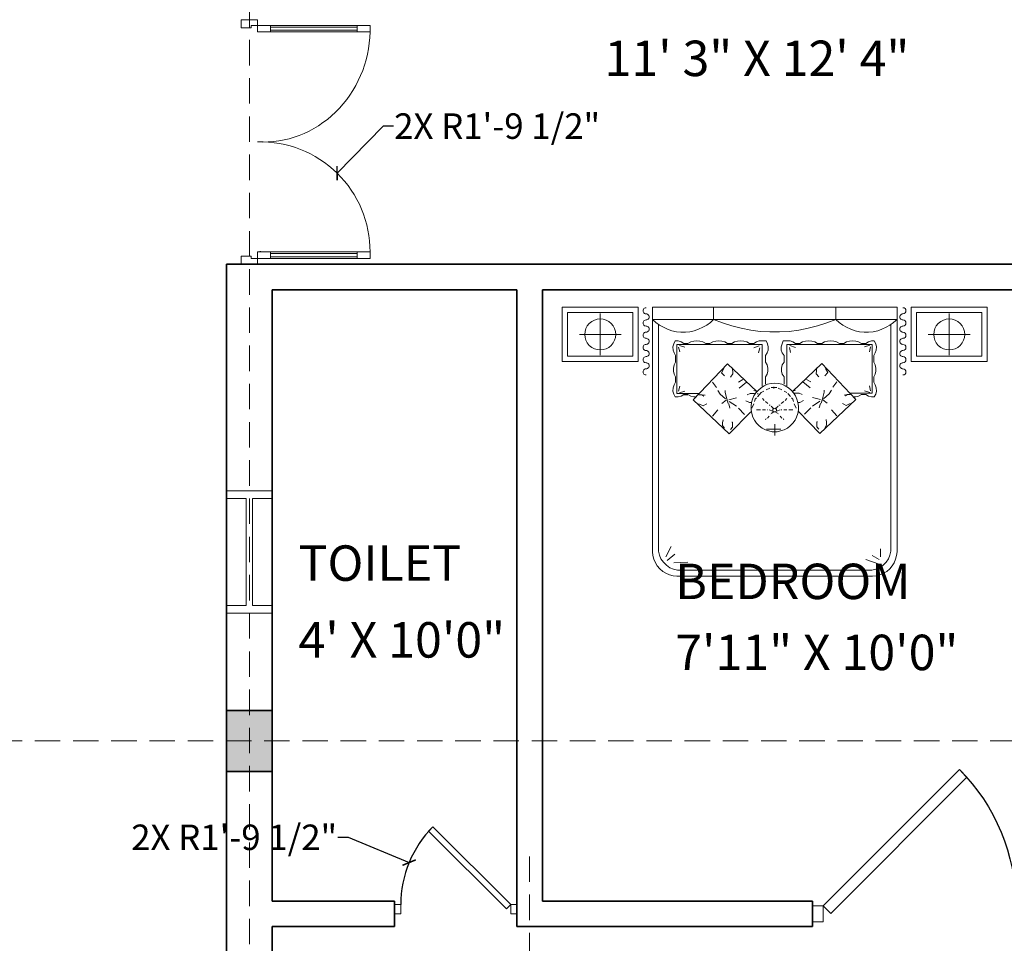
# Model space of a CAD drawing. Units: inches. Extents: x 782 to 2660, y -1008 to 166.
# Tile 4 of 12: x 1058 to 1251, y -357 to -176. Entities that reach past the tile are written whole.
import ezdxf

# ---------------------------------------------------------------- set-up
doc = ezdxf.new("R2010")
doc.units = ezdxf.units.IN
doc.header["$MEASUREMENT"] = 0
doc.linetypes.add('DASHED', pattern=[0.75, 0.5, -0.25])
for name, color, linetype, lineweight in [('A-ANNO-DIMS', 4, 'Continuous', 18), ('A-AREA-IDEN', 4, 'Continuous', 18), ('A-COLS', 7, 'Continuous', 35), ('A-Door', 150, 'Continuous', 18), ('A-FURN', 8, 'Continuous', 13), ('A-Glaz', 4, 'Continuous', 18), ('A-GRID', 8, 'DASHED', 13), ('A-WALL', 7, 'Continuous', 35)]:
    doc.layers.add(name, color=color, linetype=linetype, lineweight=lineweight)
doc.layers.add('NET 01', color=8, linetype='Continuous')
doc.styles.get("Standard").update_dxf_attribs({"font": 'arial.ttf'})
doc.dimstyles.get("Standard").update_dxf_attribs({"dimtxt": 5, "dimasz": 2, "dimexe": 0.18, "dimexo": 0.0625, "dimgap": 0.09, "dimtad": 0, "dimtih": 1, "dimtoh": 1, "dimdec": 0, "dimzin": 0, "dimdsep": 46, "dimlunit": 3, "dimtxsty": 'Standard', "dimblk": 'ARCHTICK', "dimcen": 0.09, "dimadec": 0, "dimazin": 0, "dimtfac": 1, "dimtdec": 0, "dimtofl": 0, "dimtmove": 0, "dimatfit": 3, "dimfxl": 1, "dimtolj": 1, "dimtzin": 0, "dimarcsym": 0})

# ---------------------------------------------------------------- blocks, each defined once
blk = doc.blocks.new('A$C592222DF')
at = {"layer": 'A-Door'}
for points in [[(-0.0354, -0.0354), (-0.6718, 0.601), (-0.6364, 0.6364), (0, 0)], [(-0.95, 0), (-0.95, -0.075), (-0.9, -0.075), (-0.9, 0)], [(0, 0), (0, -0.075), (0.05, -0.075), (0.05, 0)]]:
    blk.add_lwpolyline(points, close=True, dxfattribs=at)
at = {"layer": 'NET 01'}
blk.add_arc((0, 0), 0.9, 135, 180, dxfattribs=at)
blk = doc.blocks.new('A$C13CE0A17')
at = {"layer": 'A-Door'}
for p, q in [((0, 0.61), (0, 0.69)), ((0, 0.69), (0.04, 0.69)), ((0.04, 0.69), (0.04, 0.61)), ((0, 0.61), (0, 0.08)), ((0.04, 0.61), (0, 0.61)), ((0.04, 0.61), (0, 0.61)), ((0.03, 0.61), (0.01, 0.61)), ((0.04, 0.08), (0.04, 0.61)), ((0, 0.08), (0, 0)), ((0.04, 0.08), (0, 0.08)), ((0, 0.08), (0.04, 0.08)), ((0.01, 0.08), (0.03, 0.08)), ((0.04, 0), (0.04, 0.08)), ((-0.035, 0), (-0.035, -0.1)), ((0, 0), (-0.035, 0)), ((0, 0), (0.04, 0)), ((0, -0.04), (0, 0)), ((0.015, -0.04), (0, -0.04)), ((0.015, -0.05), (0.015, -0.04)), ((0.015, -0.1), (0.015, -0.05)), ((-0.035, -0.1), (0.015, -0.1))]:
    blk.add_line(p, q, dxfattribs=at)
for points in [[(1.39, 0.69), (1.39, 0.61), (1.43, 0.61), (1.43, 0.69)], [(1.39, 0.08), (1.39, 0.61), (1.43, 0.61), (1.43, 0.08)], [(1.39, 0), (1.39, 0.08), (1.43, 0.08), (1.43, 0)], [(1.43, 0), (1.465, 0), (1.465, -0.1), (1.415, -0.1), (1.415, -0.05), (1.415, -0.04), (1.43, -0.04)]]:
    blk.add_lwpolyline(points, close=True, dxfattribs=at)
blk.add_arc((1.3872, 0.017), 0.673, 89.76573, 181.44381, dxfattribs=at)
blk.add_ellipse((0.0389, 0.0511), major_axis=(0.6669, -0.1217), ratio=0.940794, start_param=0.11153, end_param=1.73917, dxfattribs=at)
at = {"layer": 'A-Glaz'}
for p, q in [((0.01, 0.61), (0.01, 0.08)), ((0.03, 0.08), (0.03, 0.61))]:
    blk.add_line(p, q, dxfattribs=at)
blk.add_lwpolyline([(1.4, 0.08), (1.4, 0.61), (1.42, 0.61), (1.42, 0.08)], close=True, dxfattribs=at)
blk = doc.blocks.new('d-bed-4')
at = {"color": 0, "linetype": 'ByBlock'}
for p, q in [((0.56, 0), (0, 0)), ((0, 0), (0, -0.4)), ((0.56, -0.4), (0.56, 0)), ((0.6639, -1.8), (0.6639, 0)), ((0.6639, 0), (2.4639, 0)), ((0.6639, 0), (2.4639, 0)), ((0.6639, -1.8), (0.6639, 0)), ((1.1139, 0), (1.1139, -0.09)), ((2.0139, 0), (2.0139, -0.09)), ((2.4639, 0), (2.4639, -1.8)), ((2.4639, 0), (2.4639, -1.8)), ((2.5679, -0.4), (2.5679, 0)), ((2.5679, 0), (3.1279, 0)), ((3.1279, 0), (3.1279, -0.4)), ((0.52, -0.04), (0.04, -0.04)), ((0.04, -0.04), (0.04, -0.36)), ((0.28, -0.0461), (0.28, -0.3539)), ((0.52, -0.36), (0.52, -0.04)), ((2.6079, -0.36), (2.6079, -0.04)), ((2.6079, -0.04), (3.0879, -0.04)), ((2.8479, -0.0461), (2.8479, -0.3539)), ((3.0879, -0.04), (3.0879, -0.36)), ((2.4639, -0.09), (0.6639, -0.09)), ((0.6639, -0.09), (0.6891, -0.1116)), ((0.6891, -0.1116), (0.7161, -0.1314)), ((0.7089, -1.7946), (0.7089, -0.1278)), ((0.7161, -0.1314), (0.7449, -0.1476)), ((1.0347, -0.1476), (1.0635, -0.1314)), ((1.0635, -0.1314), (1.0905, -0.1116)), ((1.0905, -0.1116), (1.1139, -0.09)), ((1.1139, -0.09), (1.1805, -0.1152)), ((1.1805, -0.1152), (1.2489, -0.1368)), ((1.2489, -0.1368), (1.3173, -0.1548)), ((1.8105, -0.1548), (1.8789, -0.1368)), ((1.8789, -0.1368), (1.9473, -0.1152)), ((1.9473, -0.1152), (2.0139, -0.09)), ((2.0139, -0.09), (2.0373, -0.1116)), ((2.0373, -0.1116), (2.0643, -0.1314)), ((2.0643, -0.1314), (2.0931, -0.1476)), ((2.3829, -0.1476), (2.4117, -0.1314)), ((2.4117, -0.1314), (2.4387, -0.1116)), ((2.4189, -0.1278), (2.4189, -1.7946)), ((2.4387, -0.1116), (2.4639, -0.09)), ((0.1261, -0.2), (0.4339, -0.2)), ((0.7449, -0.1476), (0.7755, -0.162)), ((0.7755, -0.162), (0.8061, -0.1728)), ((0.8061, -0.1728), (0.8403, -0.18)), ((0.8403, -0.18), (0.8727, -0.1836)), ((0.8727, -0.1836), (0.9069, -0.1836)), ((0.9069, -0.1836), (0.9393, -0.18)), ((0.9393, -0.18), (0.9717, -0.1728)), ((0.9717, -0.1728), (1.0041, -0.162)), ((1.0041, -0.162), (1.0347, -0.1476)), ((1.3173, -0.1548), (1.3875, -0.1692)), ((1.3875, -0.1692), (1.4577, -0.1782)), ((1.4577, -0.1782), (1.5279, -0.1818)), ((1.5279, -0.1818), (1.5999, -0.1818)), ((1.5999, -0.1818), (1.6701, -0.1782)), ((1.6701, -0.1782), (1.7403, -0.1692)), ((1.7403, -0.1692), (1.8105, -0.1548)), ((2.0931, -0.1476), (2.1237, -0.162)), ((2.1237, -0.162), (2.1561, -0.1728)), ((2.1561, -0.1728), (2.1885, -0.18)), ((2.1885, -0.18), (2.2209, -0.1836)), ((2.2209, -0.1836), (2.2551, -0.1836)), ((2.2551, -0.1836), (2.2875, -0.18)), ((2.2875, -0.18), (2.3217, -0.1728)), ((2.3217, -0.1728), (2.3523, -0.162)), ((2.3523, -0.162), (2.3829, -0.1476)), ((3.0018, -0.2), (2.6939, -0.2)), ((0.8151, -0.2916), (0.8205, -0.2682)), ((0.8205, -0.2682), (0.8313, -0.2484)), ((0.8313, -0.2484), (0.8529, -0.2484)), ((0.8439, -0.6354), (0.8439, -0.2754)), ((0.8439, -0.2754), (1.4721, -0.2754)), ((0.8529, -0.2484), (0.8745, -0.2556)), ((0.8619, -0.2808), (0.9015, -0.2934)), ((0.8745, -0.2556), (0.8943, -0.2664)), ((0.8943, -0.2664), (0.9249, -0.2664)), ((0.9249, -0.2664), (0.9465, -0.2556)), ((0.9465, -0.2556), (0.9681, -0.2502)), ((0.9681, -0.2502), (0.9897, -0.2484)), ((0.9897, -0.2484), (1.0131, -0.2502)), ((1.0131, -0.2502), (1.0347, -0.2556)), ((1.0347, -0.2556), (1.0563, -0.2664)), ((1.0563, -0.2664), (1.0869, -0.2664)), ((1.0869, -0.2664), (1.1085, -0.2556)), ((1.1085, -0.2556), (1.1301, -0.2502)), ((1.1301, -0.2502), (1.1517, -0.2484)), ((1.1517, -0.2484), (1.1751, -0.2502)), ((1.1751, -0.2502), (1.1967, -0.2556)), ((1.1967, -0.2556), (1.2165, -0.2664)), ((1.2165, -0.2664), (1.2489, -0.2664)), ((1.2489, -0.2664), (1.2687, -0.2556)), ((1.2687, -0.2556), (1.2903, -0.2502)), ((1.2903, -0.2502), (1.3137, -0.2484)), ((1.3137, -0.2484), (1.3371, -0.2502)), ((1.3371, -0.2502), (1.3587, -0.2556)), ((1.3587, -0.2556), (1.3785, -0.2664)), ((1.3785, -0.2664), (1.4109, -0.2664)), ((1.4505, -0.2844), (1.4091, -0.2988)), ((1.4109, -0.2664), (1.4307, -0.2556)), ((1.4307, -0.2556), (1.4505, -0.2484)), ((1.4505, -0.2484), (1.4739, -0.2484)), ((1.4721, -0.2754), (1.4721, -0.5814)), ((1.4739, -0.2484), (1.5009, -0.2484)), ((1.5009, -0.2484), (1.5099, -0.2682)), ((1.5099, -0.2682), (1.5153, -0.2916)), ((1.6179, -0.2682), (1.6125, -0.2916)), ((1.6269, -0.2484), (1.6179, -0.2682)), ((1.6539, -0.2484), (1.6269, -0.2484)), ((1.6773, -0.2484), (1.6539, -0.2484)), ((2.2821, -0.2736), (1.6539, -0.2736)), ((1.6539, -0.2736), (1.6539, -0.5796)), ((1.6755, -0.2826), (1.7169, -0.297)), ((1.6971, -0.2556), (1.6773, -0.2484)), ((1.7169, -0.2664), (1.6971, -0.2556)), ((1.7493, -0.2664), (1.7169, -0.2664)), ((1.7691, -0.2556), (1.7493, -0.2664)), ((1.7907, -0.2502), (1.7691, -0.2556)), ((1.8141, -0.2484), (1.7907, -0.2502)), ((1.8375, -0.2502), (1.8141, -0.2484)), ((1.8591, -0.2556), (1.8375, -0.2502)), ((1.8789, -0.2664), (1.8591, -0.2556)), ((1.9113, -0.2664), (1.8789, -0.2664)), ((1.9311, -0.2556), (1.9113, -0.2664)), ((1.9527, -0.2502), (1.9311, -0.2556)), ((1.9761, -0.2484), (1.9527, -0.2502)), ((1.9977, -0.2502), (1.9761, -0.2484)), ((2.0193, -0.2556), (1.9977, -0.2502)), ((2.0409, -0.2664), (2.0193, -0.2556)), ((2.0715, -0.2664), (2.0409, -0.2664)), ((2.0931, -0.2556), (2.0715, -0.2664)), ((2.1147, -0.2502), (2.0931, -0.2556)), ((2.1381, -0.2484), (2.1147, -0.2502)), ((2.1597, -0.2502), (2.1381, -0.2484)), ((2.1813, -0.2556), (2.1597, -0.2502)), ((2.2029, -0.2664), (2.1813, -0.2556)), ((2.2335, -0.2664), (2.2029, -0.2664)), ((2.2641, -0.279), (2.2245, -0.2916)), ((2.2533, -0.2556), (2.2335, -0.2664)), ((2.2749, -0.2484), (2.2533, -0.2556)), ((2.2965, -0.2484), (2.2749, -0.2484)), ((2.2821, -0.6336), (2.2821, -0.2736)), ((2.3073, -0.2682), (2.2965, -0.2484)), ((2.3127, -0.2916), (2.3073, -0.2682)), ((0.04, -0.36), (0.52, -0.36)), ((0.8169, -0.315), (0.8151, -0.2916)), ((0.8241, -0.3366), (0.8169, -0.315)), ((0.8349, -0.3564), (0.8241, -0.3366)), ((0.8349, -0.405), (0.8349, -0.3564)), ((0.8565, -0.2934), (0.8655, -0.3294)), ((1.4541, -0.2988), (1.4451, -0.3348)), ((1.5081, -0.3366), (1.4955, -0.3564)), ((1.4955, -0.3564), (1.4955, -0.405)), ((1.5153, -0.315), (1.5081, -0.3366)), ((1.5153, -0.2916), (1.5153, -0.315)), ((1.6125, -0.2916), (1.6125, -0.315)), ((1.6125, -0.315), (1.6197, -0.3366)), ((1.6197, -0.3366), (1.6323, -0.3564)), ((1.6323, -0.3564), (1.6323, -0.405)), ((1.6719, -0.297), (1.6809, -0.333)), ((2.2695, -0.2916), (2.2605, -0.3276)), ((2.2929, -0.3564), (2.3037, -0.3366)), ((2.2929, -0.405), (2.2929, -0.3564)), ((2.3037, -0.3366), (2.3109, -0.315)), ((2.3109, -0.315), (2.3127, -0.2916)), ((3.0879, -0.36), (2.6079, -0.36)), ((0, -0.4), (0.56, -0.4)), ((0.8187, -0.4482), (0.8241, -0.4248)), ((0.8241, -0.4248), (0.8349, -0.405)), ((0.9645, -0.6804), (1.2165, -0.4158)), ((1.2165, -0.4158), (1.4325, -0.621)), ((1.4955, -0.405), (1.5081, -0.4248)), ((1.5081, -0.4248), (1.5135, -0.4482)), ((1.6197, -0.4248), (1.6143, -0.4482)), ((1.6323, -0.405), (1.6197, -0.4248)), ((1.9095, -0.414), (1.6935, -0.6192)), ((2.1615, -0.6786), (1.9095, -0.414)), ((2.3037, -0.4248), (2.2929, -0.405)), ((2.3091, -0.4482), (2.3037, -0.4248)), ((3.1279, -0.4), (2.5679, -0.4)), ((0.8187, -0.4698), (0.8187, -0.4482)), ((0.8241, -0.4932), (0.8187, -0.4698)), ((0.8349, -0.513), (0.8241, -0.4932)), ((1.1895, -0.4518), (1.1715, -0.4824)), ((1.1715, -0.4824), (1.1931, -0.5058)), ((1.2561, -0.4914), (1.2381, -0.5148)), ((1.2525, -0.4464), (1.2561, -0.4914)), ((1.5081, -0.4932), (1.4955, -0.513)), ((1.5135, -0.4698), (1.5081, -0.4932)), ((1.5135, -0.4482), (1.5135, -0.4698)), ((1.6143, -0.4482), (1.6143, -0.4698)), ((1.6143, -0.4698), (1.6197, -0.4932)), ((1.6197, -0.4932), (1.6323, -0.513)), ((1.8735, -0.4446), (1.8699, -0.4896)), ((1.8699, -0.4896), (1.8879, -0.513)), ((1.9545, -0.4806), (1.9329, -0.504)), ((1.9365, -0.45), (1.9545, -0.4806)), ((2.2929, -0.513), (2.3037, -0.4932)), ((2.3037, -0.4932), (2.3091, -0.4698)), ((2.3091, -0.4698), (2.3091, -0.4482)), ((0.8169, -0.594), (0.8241, -0.5724)), ((0.8241, -0.5724), (0.8349, -0.5526)), ((0.8349, -0.5526), (0.8349, -0.513)), ((1.1049, -0.5508), (1.1355, -0.5904)), ((1.3281, -0.5328), (1.2975, -0.5508)), ((1.3551, -0.5508), (1.3011, -0.5958)), ((1.4631, -0.5922), (1.4865, -0.5778)), ((1.4865, -0.5778), (1.5117, -0.567)), ((1.4955, -0.513), (1.4955, -0.567)), ((1.5117, -0.567), (1.5369, -0.5616)), ((1.5369, -0.5616), (1.5639, -0.558)), ((1.5639, -0.558), (1.5909, -0.5616)), ((1.5909, -0.5616), (1.6161, -0.567)), ((1.6161, -0.567), (1.6413, -0.5778)), ((1.6323, -0.513), (1.6323, -0.567)), ((1.6413, -0.5778), (1.6647, -0.5922)), ((1.7709, -0.549), (1.8249, -0.594)), ((1.7979, -0.531), (1.8285, -0.549)), ((2.0211, -0.549), (1.9905, -0.5886)), ((2.2695, -0.6156), (2.2605, -0.5796)), ((2.2929, -0.5526), (2.2929, -0.513)), ((2.3037, -0.5724), (2.2929, -0.5526)), ((2.3109, -0.594), (2.3037, -0.5724)), ((0.8151, -0.6174), (0.8169, -0.594)), ((0.8205, -0.6408), (0.8151, -0.6174)), ((0.8313, -0.6606), (0.8205, -0.6408)), ((1.0095, -0.6354), (0.8439, -0.6354)), ((0.8565, -0.6174), (0.8655, -0.5814)), ((0.8619, -0.63), (0.9015, -0.6174)), ((0.8943, -0.6426), (0.8745, -0.6534)), ((0.9069, -0.6444), (0.8925, -0.6444)), ((0.9249, -0.6426), (0.8943, -0.6426)), ((0.9159, -0.6444), (0.9069, -0.6444)), ((0.9249, -0.6444), (0.9159, -0.6444)), ((0.9465, -0.6534), (0.9249, -0.6426)), ((1.0059, -0.6444), (1.0239, -0.6444)), ((1.0239, -0.6444), (1.0419, -0.6534)), ((1.0419, -0.6534), (1.0275, -0.6444)), ((1.0275, -0.6444), (1.0509, -0.648)), ((1.1625, -0.639), (1.1445, -0.612)), ((1.2021, -0.675), (1.1625, -0.639)), ((1.1985, -0.6264), (1.1985, -0.612)), ((1.2111, -0.675), (1.1985, -0.6264)), ((1.3821, -0.6354), (1.3605, -0.6444)), ((1.4145, -0.6354), (1.3821, -0.6354)), ((1.4001, -0.6768), (1.4109, -0.6516)), ((1.4091, -0.612), (1.4325, -0.621)), ((1.4109, -0.6516), (1.4253, -0.63)), ((1.4145, -0.6354), (1.4181, -0.639)), ((1.4253, -0.63), (1.4433, -0.6102)), ((1.4649, -0.6264), (1.4379, -0.6588)), ((1.4379, -0.6354), (1.4415, -0.6408)), ((1.4433, -0.6102), (1.4631, -0.5922)), ((1.4649, -0.6264), (1.4829, -0.6174)), ((1.5279, -0.5958), (1.5009, -0.6084)), ((1.5369, -0.5904), (1.5621, -0.5904)), ((1.5801, -0.5904), (1.5549, -0.5904)), ((1.5585, -0.5868), (1.5585, -0.5994)), ((1.5585, -0.5868), (1.5585, -0.5994)), ((1.5891, -0.5958), (1.6161, -0.6084)), ((1.6521, -0.6264), (1.6341, -0.6174)), ((1.6593, -0.6354), (1.6809, -0.657)), ((1.6647, -0.5922), (1.6845, -0.6102)), ((1.6845, -0.6102), (1.7025, -0.63)), ((1.7169, -0.6102), (1.6935, -0.6192)), ((1.7025, -0.63), (1.7169, -0.6516)), ((1.7115, -0.6336), (1.7079, -0.6372)), ((1.7115, -0.6336), (1.7439, -0.6336)), ((1.7169, -0.6516), (1.7277, -0.6768)), ((1.7439, -0.6336), (1.7655, -0.6426)), ((1.9149, -0.6732), (1.9275, -0.6246)), ((1.9239, -0.6732), (1.9635, -0.6372)), ((1.9275, -0.6246), (1.9275, -0.6102)), ((1.9635, -0.6372), (1.9815, -0.6102)), ((2.0985, -0.6426), (2.0751, -0.6462)), ((2.1021, -0.6426), (2.0841, -0.6516)), ((2.0841, -0.6516), (2.0985, -0.6426)), ((2.1201, -0.6426), (2.1021, -0.6426)), ((2.1165, -0.6336), (2.2821, -0.6336)), ((2.1813, -0.6534), (2.2029, -0.6426)), ((2.2011, -0.6426), (2.2101, -0.6426)), ((2.2029, -0.6426), (2.2335, -0.6426)), ((2.2101, -0.6426), (2.2191, -0.6426)), ((2.2191, -0.6426), (2.2335, -0.6426)), ((2.2641, -0.6282), (2.2245, -0.6156)), ((2.2335, -0.6426), (2.2533, -0.6534)), ((2.2965, -0.6606), (2.3073, -0.6408)), ((2.3073, -0.6408), (2.3127, -0.6174)), ((2.3127, -0.6174), (2.3109, -0.594)), ((0.8529, -0.6606), (0.8313, -0.6606)), ((0.8745, -0.6534), (0.8529, -0.6606)), ((0.9681, -0.6588), (0.9465, -0.6534)), ((1.2291, -0.9324), (0.9645, -0.6804)), ((0.9825, -0.6606), (0.9681, -0.6588)), ((1.0059, -0.711), (1.0365, -0.7254)), ((1.0365, -0.7254), (1.0545, -0.7164)), ((1.0545, -0.7164), (1.0635, -0.711)), ((1.1751, -0.7074), (1.2075, -0.684)), ((1.2201, -0.7074), (1.2111, -0.675)), ((1.2255, -0.6804), (1.2831, -0.666)), ((1.2255, -0.711), (1.2345, -0.7434)), ((1.2291, -0.693), (1.2831, -0.729)), ((1.3785, -0.702), (1.3515, -0.6894)), ((1.3785, -0.702), (1.3911, -0.702)), ((1.3893, -0.729), (1.3929, -0.702)), ((1.3929, -0.702), (1.4001, -0.6768)), ((1.3965, -0.7434), (1.4109, -0.711)), ((1.4199, -0.6768), (1.4145, -0.6948)), ((1.4199, -0.6768), (1.4289, -0.6678)), ((1.4865, -0.6858), (1.4739, -0.6714)), ((1.5135, -0.7074), (1.4955, -0.6948)), ((1.5315, -0.72), (1.5225, -0.72)), ((1.5945, -0.72), (1.6035, -0.72)), ((1.6125, -0.7074), (1.6305, -0.6948)), ((1.6395, -0.6858), (1.6521, -0.6714)), ((1.6971, -0.6768), (1.6881, -0.6678)), ((1.6971, -0.6768), (1.7025, -0.6948)), ((1.7205, -0.7434), (1.7061, -0.711)), ((1.7277, -0.6768), (1.7349, -0.702)), ((1.7475, -0.7002), (1.7349, -0.7002)), ((1.7349, -0.702), (1.7385, -0.729)), ((1.7475, -0.7002), (1.7745, -0.6876)), ((1.9005, -0.6786), (1.8429, -0.6642)), ((1.8969, -0.6912), (1.8429, -0.7272)), ((1.9005, -0.7092), (1.8915, -0.7416)), ((1.8969, -0.9306), (2.1615, -0.6786)), ((1.9059, -0.7056), (1.9149, -0.6732)), ((1.9509, -0.7056), (1.9185, -0.6822)), ((2.0715, -0.7146), (2.0625, -0.7092)), ((2.0895, -0.7236), (2.0715, -0.7146)), ((2.1201, -0.7092), (2.0895, -0.7236)), ((2.1453, -0.6606), (2.1597, -0.6588)), ((2.1597, -0.6588), (2.1813, -0.6534)), ((2.2533, -0.6534), (2.2749, -0.6606)), ((2.2749, -0.6606), (2.2965, -0.6606)), ((1.1049, -0.801), (1.1445, -0.756)), ((1.2291, -0.9324), (1.3875, -0.7704)), ((1.3425, -0.7884), (1.2975, -0.7434)), ((1.3893, -0.756), (1.3893, -0.729)), ((1.3947, -0.7812), (1.3893, -0.756)), ((1.4037, -0.8082), (1.3947, -0.7812)), ((1.4595, -0.756), (1.4289, -0.756)), ((1.4955, -0.756), (1.4739, -0.756)), ((1.5135, -0.756), (1.5099, -0.756)), ((1.5495, -0.765), (1.5225, -0.756)), ((1.5315, -0.792), (1.5315, -0.792)), ((1.5585, -0.747), (1.5369, -0.729)), ((1.5585, -0.7704), (1.5369, -0.783)), ((1.5495, -0.756), (1.5495, -0.747)), ((1.5495, -0.747), (1.5585, -0.747)), ((1.5495, -0.765), (1.5495, -0.756)), ((1.5585, -0.7704), (1.5495, -0.765)), ((1.5585, -0.747), (1.5621, -0.7452)), ((1.5585, -0.7704), (1.5621, -0.7704)), ((1.5675, -0.747), (1.5621, -0.7452)), ((1.5675, -0.7704), (1.5621, -0.7704)), ((1.5675, -0.747), (1.5891, -0.729)), ((1.5765, -0.747), (1.5675, -0.747)), ((1.5675, -0.7704), (1.5765, -0.765)), ((1.5675, -0.7704), (1.5891, -0.783)), ((1.5765, -0.756), (1.5765, -0.747)), ((1.5765, -0.765), (1.5765, -0.756)), ((1.5765, -0.765), (1.6035, -0.756)), ((1.5945, -0.792), (1.5945, -0.792)), ((1.6125, -0.756), (1.6161, -0.756)), ((1.6305, -0.756), (1.6521, -0.756)), ((1.6665, -0.756), (1.6971, -0.756)), ((1.7331, -0.7812), (1.7241, -0.8082)), ((1.7385, -0.756), (1.7331, -0.7812)), ((1.7385, -0.729), (1.7385, -0.756)), ((1.8969, -0.9306), (1.7385, -0.7686)), ((1.7835, -0.7866), (1.8285, -0.7416)), ((2.0211, -0.7992), (1.9815, -0.7542)), ((1.1805, -0.8514), (1.1841, -0.828)), ((1.1805, -0.8694), (1.1805, -0.8514)), ((1.1931, -0.891), (1.1805, -0.8694)), ((1.2525, -0.846), (1.2471, -0.846)), ((1.2525, -0.882), (1.2525, -0.846)), ((1.4145, -0.8316), (1.4037, -0.8082)), ((1.4307, -0.8532), (1.4145, -0.8316)), ((1.4505, -0.873), (1.4307, -0.8532)), ((1.5009, -0.819), (1.4955, -0.828)), ((1.5225, -0.801), (1.5099, -0.8154)), ((1.5639, -0.945), (1.5639, -0.8604)), ((1.6035, -0.801), (1.6161, -0.8154)), ((1.6251, -0.819), (1.6305, -0.828)), ((1.6971, -0.8532), (1.6773, -0.873)), ((1.7133, -0.8316), (1.6971, -0.8532)), ((1.7241, -0.8082), (1.7133, -0.8316)), ((1.8735, -0.8802), (1.8735, -0.8442)), ((1.8735, -0.8442), (1.8789, -0.8442)), ((1.9329, -0.8892), (1.9455, -0.8676)), ((1.9455, -0.8496), (1.9419, -0.8262)), ((1.9455, -0.8676), (1.9455, -0.8496)), ((1.2381, -0.9), (1.2525, -0.882)), ((1.4703, -0.8892), (1.4505, -0.873)), ((1.4955, -0.9018), (1.4703, -0.8892)), ((1.5207, -0.9108), (1.4955, -0.9018)), ((1.6089, -0.8964), (1.5027, -0.8964)), ((1.5459, -0.9162), (1.5207, -0.9108)), ((1.5639, -0.9162), (1.5459, -0.9162)), ((1.5819, -0.9162), (1.5639, -0.9162)), ((1.6071, -0.9108), (1.5819, -0.9162)), ((1.6323, -0.9018), (1.6071, -0.9108)), ((1.6575, -0.8892), (1.6323, -0.9018)), ((1.6773, -0.873), (1.6575, -0.8892)), ((1.8879, -0.8982), (1.8735, -0.8802)), ((0.6675, -1.827), (0.6639, -1.8)), ((0.6675, -1.827), (0.6639, -1.8)), ((0.7161, -1.8252), (0.7089, -1.7946)), ((0.7629, -1.836), (0.8025, -1.7604)), ((2.3415, -1.836), (2.3415, -1.7784)), ((2.4189, -1.7946), (2.4117, -1.8252)), ((2.4639, -1.8), (2.4603, -1.827)), ((2.4639, -1.8), (2.4603, -1.827)), ((0.6747, -1.854), (0.6675, -1.827)), ((0.6747, -1.854), (0.6675, -1.827)), ((0.6855, -1.881), (0.6747, -1.854)), ((0.6855, -1.881), (0.6747, -1.854)), ((0.6999, -1.9044), (0.6855, -1.881)), ((0.6999, -1.9044), (0.6855, -1.881)), ((0.7269, -1.8522), (0.7161, -1.8252)), ((0.7449, -1.8774), (0.7269, -1.8522)), ((0.7665, -1.899), (0.7449, -1.8774)), ((0.7719, -1.863), (0.8295, -1.818)), ((0.8205, -1.881), (0.9249, -1.8756)), ((2.3325, -1.89), (2.2335, -1.8576)), ((2.3325, -1.8576), (2.2821, -1.827)), ((2.3829, -1.8774), (2.3613, -1.899)), ((2.4009, -1.8522), (2.3829, -1.8774)), ((2.4117, -1.8252), (2.4009, -1.8522)), ((2.4423, -1.881), (2.4279, -1.9044)), ((2.4423, -1.881), (2.4279, -1.9044)), ((2.4531, -1.854), (2.4423, -1.881)), ((2.4531, -1.854), (2.4423, -1.881)), ((2.4603, -1.827), (2.4531, -1.854)), ((2.4603, -1.827), (2.4531, -1.854)), ((0.7179, -1.926), (0.6999, -1.9044)), ((0.7179, -1.926), (0.6999, -1.9044)), ((0.7395, -1.944), (0.7179, -1.926)), ((0.7395, -1.944), (0.7179, -1.926)), ((0.7629, -1.9584), (0.7395, -1.944)), ((0.7629, -1.9584), (0.7395, -1.944)), ((0.7917, -1.917), (0.7665, -1.899)), ((0.8187, -1.9278), (0.7917, -1.917)), ((0.8493, -1.935), (0.8187, -1.9278)), ((2.2785, -1.935), (0.8493, -1.935)), ((2.3091, -1.9278), (2.2785, -1.935)), ((2.3361, -1.917), (2.3091, -1.9278)), ((2.3613, -1.899), (2.3361, -1.917)), ((2.3883, -1.944), (2.3649, -1.9584)), ((2.3883, -1.944), (2.3649, -1.9584)), ((2.4099, -1.926), (2.3883, -1.944)), ((2.4099, -1.926), (2.3883, -1.944)), ((2.4279, -1.9044), (2.4099, -1.926)), ((2.4279, -1.9044), (2.4099, -1.926)), ((0.7899, -1.9692), (0.7629, -1.9584)), ((0.7899, -1.9692), (0.7629, -1.9584)), ((0.8169, -1.9764), (0.7899, -1.9692)), ((0.8169, -1.9764), (0.7899, -1.9692)), ((0.8439, -1.98), (0.8169, -1.9764)), ((0.8439, -1.98), (0.8169, -1.9764)), ((2.2839, -1.98), (0.8439, -1.98)), ((2.2839, -1.98), (0.8439, -1.98)), ((2.3109, -1.9764), (2.2839, -1.98)), ((2.3109, -1.9764), (2.2839, -1.98)), ((2.3379, -1.9692), (2.3109, -1.9764)), ((2.3379, -1.9692), (2.3109, -1.9764)), ((2.3649, -1.9584), (2.3379, -1.9692)), ((2.3649, -1.9584), (2.3379, -1.9692))]:
    blk.add_line(p, q, dxfattribs=at)
for centre, major_axis, start_param, end_param in [((0.6172, -0.0263), (-0.0159, 0.0159), 5.497787, 8.63938), ((0.6172, -0.0713), (-0.0159, 0.0159), 2.356194, 5.497787), ((2.5072, -0.0713), (0.0159, 0.0159), 0.785398, 3.926991), ((2.5072, -0.0263), (0.0159, 0.0159), 3.926991, 7.068583), ((0.6172, -0.1163), (-0.0159, 0.0159), 5.497787, 8.63938), ((0.6172, -0.1613), (-0.0159, 0.0159), 2.356194, 5.497787), ((0.6172, -0.1613), (-0.0159, 0.0159), 2.356194, 5.497787), ((2.5072, -0.1613), (0.0159, 0.0159), 0.785398, 3.926991), ((2.5072, -0.1613), (0.0159, 0.0159), 0.785398, 3.926991), ((2.5072, -0.1163), (0.0159, 0.0159), 3.926991, 7.068583), ((0.6172, -0.2063), (-0.0159, 0.0159), 5.497787, 8.63938), ((2.5072, -0.2063), (0.0159, 0.0159), 3.926991, 7.068583), ((0.6172, -0.2963), (-0.0159, 0.0159), 5.497787, 8.63938), ((0.6172, -0.2513), (-0.0159, 0.0159), 2.356194, 5.497787), ((2.5072, -0.2513), (0.0159, 0.0159), 0.785398, 3.926991), ((2.5072, -0.2963), (0.0159, 0.0159), 3.926991, 7.068583), ((0.6172, -0.3413), (-0.0159, 0.0159), 2.356194, 5.497787), ((2.5072, -0.3413), (0.0159, 0.0159), 0.785398, 3.926991), ((0.6172, -0.3863), (-0.0159, 0.0159), 5.497787, 8.63938), ((0.6172, -0.4313), (-0.0159, 0.0159), 2.356194, 5.497787), ((2.5072, -0.4313), (0.0159, 0.0159), 0.785398, 3.926991), ((2.5072, -0.3863), (0.0159, 0.0159), 3.926991, 7.068583), ((0.6172, -0.4763), (-0.0159, 0.0159), 5.497787, 8.63938), ((2.5072, -0.4763), (0.0159, 0.0159), 3.926991, 7.068583)]:
    blk.add_ellipse(centre, major_axis=major_axis, ratio=1, start_param=start_param, end_param=end_param, dxfattribs=at)
for centre in [(0.28, -0.2), (2.8479, -0.2)]:
    blk.add_ellipse(centre, major_axis=(-0.0806, 0.0806), ratio=1, dxfattribs=at)
blk = doc.blocks.new('WIN-24')
for p, q in [((0, 0), (0, 24)), ((0, 24), (9, 24)), ((9, 24), (9, 0)), ((0, 22.49), (3.9, 22.49)), ((3.9, 1.51), (3.9, 22.49)), ((5.1, 22.49), (9, 22.49)), ((5.1, 1.51), (5.1, 22.49)), ((3.9, 1.51), (0, 1.51)), ((9, 0), (0, 0)), ((9, 1.51), (5.1, 1.51))]:
    blk.add_line(p, q)
blk = doc.blocks.new('COL-9X12')
h = blk.add_hatch(color=256)
h.dxf.hatch_style = 1
h.paths.add_polyline_path([(9, 12), (0, 12), (0, 0), (9, 0)])
blk.add_lwpolyline([(0, 12), (9, 12), (9, 0), (0, 0)], close=True)
blk = doc.blocks.new('_ArchTick')
at = {"color": 0, "linetype": 'ByBlock', "const_width": 0.15}
blk.add_lwpolyline([(-0.5, -0.5), (0.5, 0.5)], dxfattribs=at)
blk = doc.blocks.new('*D62')
at = {"layer": 'A-ANNO-DIMS', "color": 0, "lineweight": -2, "transparency": 16777216}
for p, q in [((1120.55, -336.47), (1122.55, -336.47)), ((1122.55, -336.47), (1134.53, -341.43)), ((1154.39, -349.69), (1154.57, -349.69)), ((1154.48, -349.78), (1154.48, -349.6))]:
    blk.add_line(p, q, dxfattribs=at)
at = {"layer": 'Defpoints', "color": 0, "transparency": 16777216}
for p in [(1134.53, -341.43), (1154.48, -349.69)]:
    blk.add_point(p, dxfattribs=at)
at = {"layer": 'A-ANNO-DIMS', "color": 0, "lineweight": -2, "transparency": 16777216, "xscale": 2, "yscale": 2, "zscale": 2, "rotation": 337.5006319607729}
blk.add_blockref('_ArchTick', (1134.53, -341.43), dxfattribs=at)
at = {"layer": 'A-ANNO-DIMS', "color": 0, "transparency": 16777216, "insert": (1100.19, -336.47), "char_height": 5, "attachment_point": 5}
blk.add_mtext('\\A1;2X R1\'-9 1/2"', dxfattribs=at)
blk = doc.blocks.new('*D63')
at = {"layer": 'A-ANNO-DIMS', "color": 0, "lineweight": -2, "transparency": 16777216}
for p, q in [((1129.43, -196.88), (1120.39, -206.12)), ((1131.43, -196.88), (1129.43, -196.88)), ((1105.24, -221.51), (1105.42, -221.51)), ((1105.33, -221.6), (1105.33, -221.42))]:
    blk.add_line(p, q, dxfattribs=at)
at = {"layer": 'Defpoints', "color": 0, "transparency": 16777216}
for p in [(1120.39, -206.12), (1105.33, -221.51)]:
    blk.add_point(p, dxfattribs=at)
at = {"layer": 'A-ANNO-DIMS', "color": 0, "lineweight": -2, "transparency": 16777216, "xscale": 2, "yscale": 2, "zscale": 2, "rotation": 225.6055584287821}
blk.add_blockref('_ArchTick', (1120.39, -206.12), dxfattribs=at)
at = {"layer": 'A-ANNO-DIMS', "color": 0, "transparency": 16777216, "insert": (1151.8, -196.88), "char_height": 5, "attachment_point": 5}
blk.add_mtext('\\A1;2X R1\'-9 1/2"', dxfattribs=at)

msp = doc.modelspace()

# ---------------------------------------------------------------- linework, layer by layer
at = {"layer": 'A-GRID', "ltscale": 10}
for p, q in [((1103.18, 82.53), (1103.18, -946.37)), ((866.08, -317.56), (1499.56, -317.56)), ((1158.18, -340.22), (1158.18, -911.03))]:
    msp.add_line(p, q, dxfattribs=at)
at = {"layer": 'A-WALL'}
for p, q in [((1107.68, -223.99), (1098.68, -223.99)), ((1098.68, -223.99), (1098.68, -428.99)), ((1107.68, -223.99), (1255.68, -223.99)), ((1107.68, -228.99), (1107.68, -348.99)), ((1107.68, -228.99), (1155.68, -228.99)), ((1155.68, -228.99), (1155.68, -348.99)), ((1160.68, -228.99), (1160.68, -348.99)), ((1160.68, -228.99), (1255.68, -228.99)), ((1107.68, -348.99), (1131.68, -348.99)), ((1131.68, -348.99), (1131.68, -353.99)), ((1155.68, -348.99), (1155.68, -353.99)), ((1160.68, -348.99), (1213.68, -348.99)), ((1213.68, -348.99), (1213.68, -353.99)), ((1107.68, -353.99), (1107.68, -428.99)), ((1107.68, -353.99), (1131.68, -353.99)), ((1155.68, -353.99), (1213.68, -353.99))]:
    msp.add_line(p, q, dxfattribs=at)

# ---------------------------------------------------------------- block references
at = {"layer": 'A-COLS', "rotation": 180}
msp.add_blockref('COL-9X12', (1107.68, -311.56), dxfattribs=at)
at = {"layer": 'A-Door', "xscale": 32, "yscale": 32, "zscale": 32, "rotation": 270}
msp.add_blockref('A$C13CE0A17', (1104.78, -177.11), dxfattribs=at)
at = {"layer": 'A-Door'}
for p, xscale, yscale, zscale in [((1215.78, -349.92), -42, 42, 42), ((1154.48, -349.69), 24, 24, 24)]:
    msp.add_blockref('A$C592222DF', p, dxfattribs=dict(at, xscale=xscale, yscale=yscale, zscale=zscale))
at = {"layer": 'A-FURN', "xscale": 26.66666775212405, "yscale": 26.66666775212405, "zscale": 26.66666775212405}
msp.add_blockref('d-bed-4', (1164.57, -232.43), dxfattribs=at)
at = {"layer": 'A-Glaz'}
msp.add_blockref('WIN-24', (1098.68, -292.46), dxfattribs=at)

# ---------------------------------------------------------------- texts
at = {"layer": 'A-AREA-IDEN'}
for s, height, p in [('11\' 3" X 12\' 4"', 6.9576, (1172.87, -187.06)), ('TOILET', 6.958, (1112.82, -286.13)), ('BEDROOM', 6.958, (1186.74, -289.72)), ('4\' X 10\'0"', 6.958, (1112.82, -301.2)), ('7\'11" X 10\'0"', 6.9576, (1186.74, -303.66))]:
    msp.add_text(s, height=height, dxfattribs=at).set_placement(p)

# ---------------------------------------------------------------- dimensions: what is measured, and where the dimension line sits
at = {"layer": 'A-ANNO-DIMS'}
for center, mpoint, picture, middle in [((1105.33, -221.51), (1120.39, -206.12), '*D63', (1151.8, -196.88)), ((1154.48, -349.69), (1134.53, -341.43), '*D62', (1100.19, -336.47))]:
    dim = msp.add_radius_dim(center=center, mpoint=mpoint, text='2X <>', dimstyle='Standard', override={"dimdec": 1, "dimlfac": 1, "dimrnd": 0, "dimzin": 1, "dimdsep": 46, "dimlunit": 4, "dimfrac": 2}, dxfattribs=at)
    dim.commit()
    dim.dimension.update_dxf_attribs({"geometry": picture, "text_midpoint": middle, "dimtype": 164})

doc.saveas('drawing.dxf')
